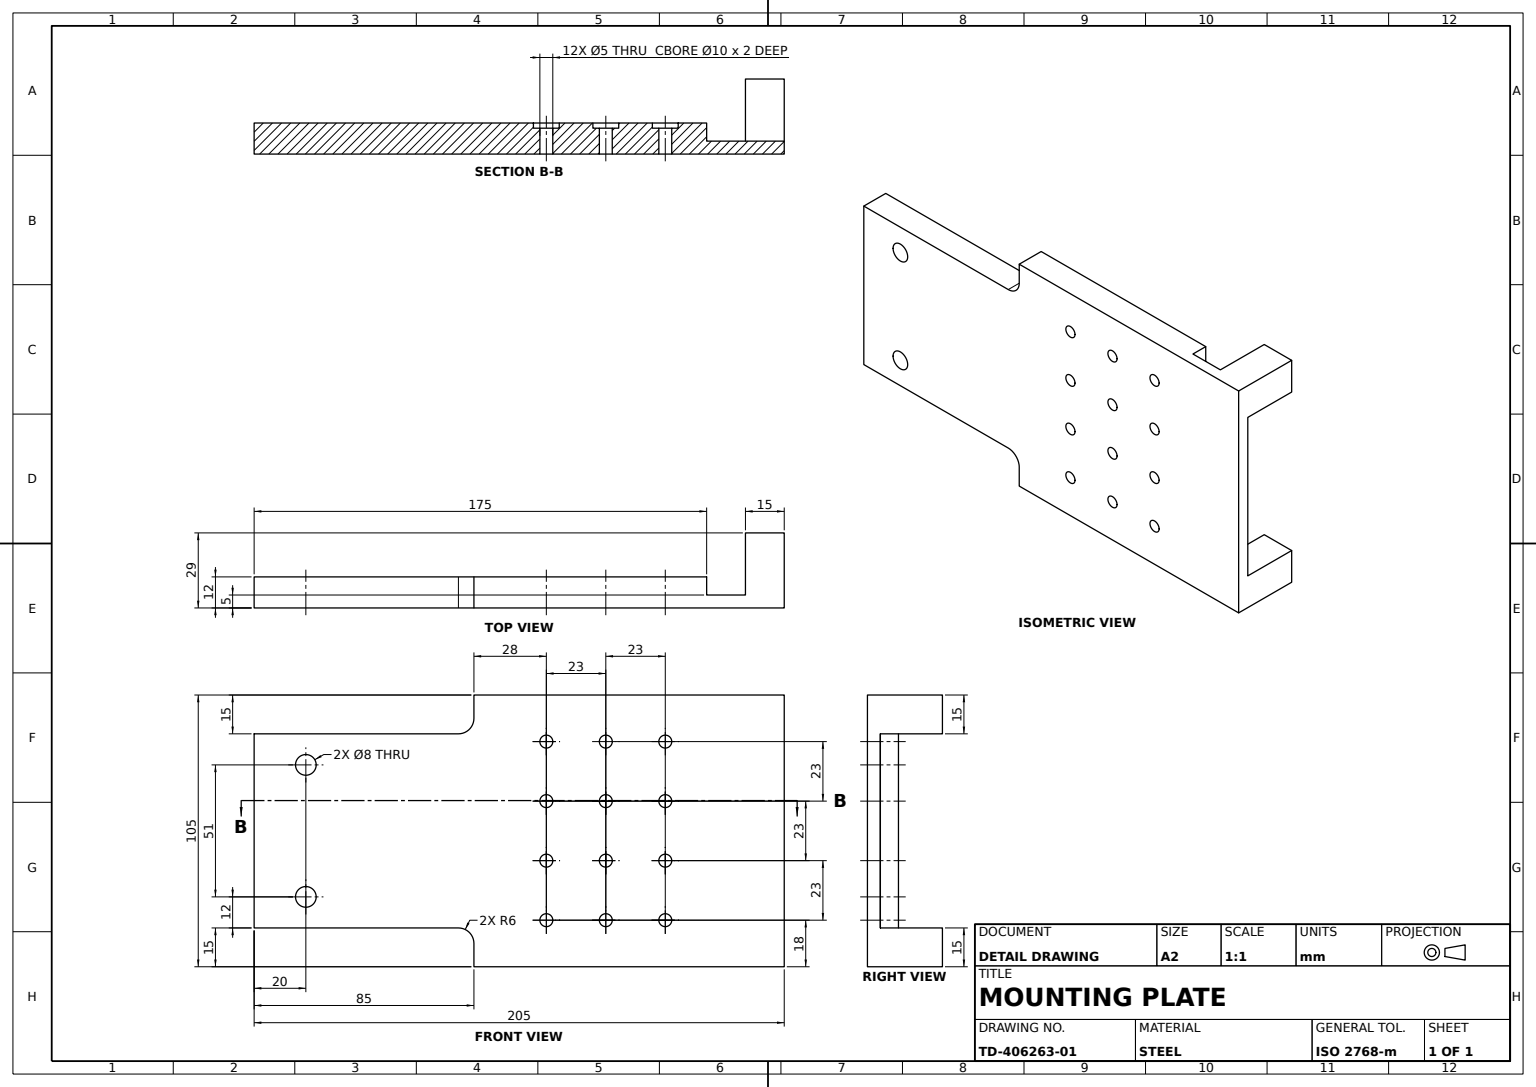
from build123d import *

# Parameters (mm, degrees)
BASE_PLATE_SKETCH_W       = 85
BASE_PLATE_SKETCH_H       = 75
BASE_PLATE_85X75_DEPTH    = 12
PLATE_EXTENSION_DEPTH     = 12
NOTCH_FILLET_R6_A_R       = 6
NOTCH_FILLET_R6_B_R       = 6
END_FLANGE_SKETCH_W       = 30
END_FLANGE_SKETCH_H       = 105
END_FLANGE_DEPTH          = 5
SIDE_TAB_1_SKETCH_W       = 15
SIDE_TAB_1_SKETCH_H       = 24
SIDE_TAB_1_DEPTH          = 15
SIDE_TAB_2_SKETCH_W       = 15
SIDE_TAB_2_SKETCH_H       = 24
SIDE_TAB_2_DEPTH          = 15
COUNTERBORE_GRID_SKETCH_R = 5
COUNTERBORES_12X_10_DEPTH = 2
HOLE_GRID_SKETCH_R        = 2.5
HOLE_GRID_12X_5_DEPTH     = 10
MOUNTING_HOLES_SKETCH_R   = 4
MOUNTING_HOLES_2X_8_DEPTH = 15


with BuildPart() as part:
    # Base Plate Sketch → Base Plate 85x75 (new body)
    with BuildSketch(Plane.XY):
        with Locations((42.5, 37.5)):
            Rectangle(BASE_PLATE_SKETCH_W, BASE_PLATE_SKETCH_H)
    extrude(amount=BASE_PLATE_85X75_DEPTH)

    # Plate Extension Sketch → Plate Extension (add)
    with BuildSketch(Plane.XY.offset(12)):
        Polygon((85, 75), (85, 37.5), (175, 37.5), (175, 90), (85, 90), align=None)
        Polygon((175, 37.5), (85, 37.5), (85, 0), (85, -15), (175, -15), align=None)
    extrude(amount=-PLATE_EXTENSION_DEPTH)

    # Notch Fillet R6 A
    notch_fillet_r6_a_edges = [part.edges().sort_by_distance(p)[0] for p in [
        (85, 75, 6),
    ]]
    fillet(notch_fillet_r6_a_edges, radius=NOTCH_FILLET_R6_A_R)

    # Notch Fillet R6 B
    notch_fillet_r6_b_edges = [part.edges().sort_by_distance(p)[0] for p in [
        (85, 0, 6),
    ]]
    fillet(notch_fillet_r6_b_edges, radius=NOTCH_FILLET_R6_B_R)

    # End Flange Sketch → End Flange (add)
    with BuildSketch(Plane.XY.offset(12)):
        with Locations((190, 37.5)):
            Rectangle(END_FLANGE_SKETCH_W, END_FLANGE_SKETCH_H)
    extrude(amount=-END_FLANGE_DEPTH)

    # Side Tab 1 Sketch → Side Tab 1 (add)
    with BuildSketch(Plane(origin=(0, 90, 0), x_dir=(1, 0, 0), z_dir=(0, 1, 0))):
        with Locations((197.5, 5)):
            Rectangle(SIDE_TAB_1_SKETCH_W, SIDE_TAB_1_SKETCH_H)
    extrude(amount=-SIDE_TAB_1_DEPTH)

    # Side Tab 2 Sketch → Side Tab 2 (add)
    with BuildSketch(Plane.XZ.offset(15)):
        with Locations((197.5, -5)):
            Rectangle(SIDE_TAB_2_SKETCH_W, SIDE_TAB_2_SKETCH_H)
    extrude(amount=-SIDE_TAB_2_DEPTH)

    # Counterbore Grid Sketch → Counterbores 12xØ10 (cut)
    with BuildSketch(Plane(origin=(0, 0, 0), x_dir=(-1, 0, 0), z_dir=(0, 0, -1))):
        with Locations((-159, 72)):
            Circle(COUNTERBORE_GRID_SKETCH_R)
        with Locations((-136, 72)):
            Circle(COUNTERBORE_GRID_SKETCH_R)
        with Locations((-113, 72)):
            Circle(COUNTERBORE_GRID_SKETCH_R)
        with Locations((-113, 49)):
            Circle(COUNTERBORE_GRID_SKETCH_R)
        with Locations((-136, 49)):
            Circle(COUNTERBORE_GRID_SKETCH_R)
        with Locations((-159, 49)):
            Circle(COUNTERBORE_GRID_SKETCH_R)
        with Locations((-159, 26)):
            Circle(COUNTERBORE_GRID_SKETCH_R)
        with Locations((-136, 26)):
            Circle(COUNTERBORE_GRID_SKETCH_R)
        with Locations((-113, 26)):
            Circle(COUNTERBORE_GRID_SKETCH_R)
        with Locations((-113, 3)):
            Circle(COUNTERBORE_GRID_SKETCH_R)
        with Locations((-136, 3)):
            Circle(COUNTERBORE_GRID_SKETCH_R)
        with Locations((-159, 3)):
            Circle(COUNTERBORE_GRID_SKETCH_R)
    extrude(amount=-COUNTERBORES_12X_10_DEPTH, mode=Mode.SUBTRACT)

    # Hole Grid Sketch → Hole Grid 12xØ5 (cut)
    with BuildSketch(Plane(origin=(0, 0, 2), x_dir=(-1, 0, 0), z_dir=(0, 0, -1))):
        with Locations((-159, 72)):
            Circle(HOLE_GRID_SKETCH_R)
        with Locations((-136, 72)):
            Circle(HOLE_GRID_SKETCH_R)
        with Locations((-113, 72)):
            Circle(HOLE_GRID_SKETCH_R)
        with Locations((-113, 49)):
            Circle(HOLE_GRID_SKETCH_R)
        with Locations((-136, 49)):
            Circle(HOLE_GRID_SKETCH_R)
        with Locations((-159, 49)):
            Circle(HOLE_GRID_SKETCH_R)
        with Locations((-159, 26)):
            Circle(HOLE_GRID_SKETCH_R)
        with Locations((-136, 26)):
            Circle(HOLE_GRID_SKETCH_R)
        with Locations((-113, 26)):
            Circle(HOLE_GRID_SKETCH_R)
        with Locations((-159, 3)):
            Circle(HOLE_GRID_SKETCH_R)
        with Locations((-136, 3)):
            Circle(HOLE_GRID_SKETCH_R)
        with Locations((-113, 3)):
            Circle(HOLE_GRID_SKETCH_R)
    extrude(amount=-HOLE_GRID_12X_5_DEPTH, mode=Mode.SUBTRACT)

    # Mounting Holes Sketch → Mounting Holes 2xØ8 (cut)
    with BuildSketch(Plane(origin=(0, 0, 0), x_dir=(-1, 0, 0), z_dir=(0, 0, -1))):
        with Locations((-20, 63)):
            Circle(MOUNTING_HOLES_SKETCH_R)
        with Locations((-20, 12)):
            Circle(MOUNTING_HOLES_SKETCH_R)
    extrude(amount=-MOUNTING_HOLES_2X_8_DEPTH, mode=Mode.SUBTRACT)


solid = part.part
